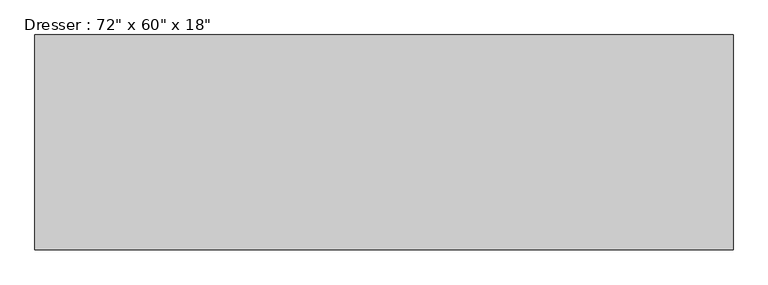
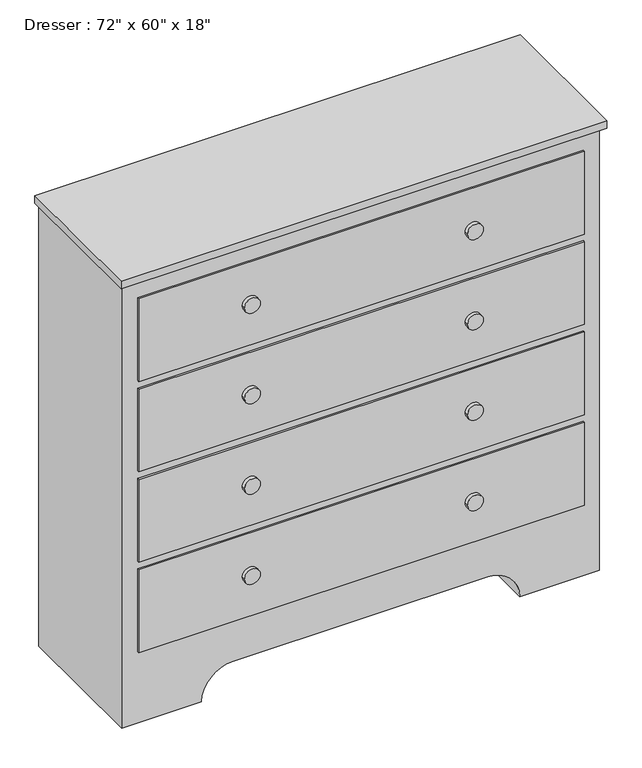
"""IFC4 building model written with IfcOpenShell, lengths in millimetres: furniture geometry."""

from ifc_helpers import new_model, si_unit, point, frame, frame_2d, origin, place, context, project, spatial, polyline, circle_curve, trimmed, segment, composite_curve, outline, extrude, source, transform, mapped, element, save


def furniture_06d35bcb(model_context):
    return source(origin(), model_context, "Body", "SweptSolid", [
        extrude(outline(polyline([(505.5067402, -134.5629541), (505.5067402, -610.8129541), (-1043.8932598, -610.8129541), (-1043.8932598, -134.5629541), (505.5067402, -134.5629541)])), frame((0.0, 0.0, 1498.6), z_axis=(0.0, 0.0, 1.0), x_axis=(1.0, 0.0, 0.0)), (0.0, 0.0, 1.0), 25.4),
        extrude(outline(composite_curve([segment(polyline([(0.0, 492.8067402), (1498.6, 492.8067402), (1498.6, -1031.1932598), (0.0, -1031.1932598), (0.0, -777.1932598)]), True, "CONTINUOUS"), segment(trimmed(circle_curve(frame_2d((0.0, -675.5932598)), 101.6), [point((0.0, -777.1932598))], [point((101.6, -675.5932598))], True, "CARTESIAN"), True, "CONTINUOUS"), segment(polyline([(101.6, -675.5932598), (101.6, 137.2067402)]), True, "CONTINUOUS"), segment(trimmed(circle_curve(frame_2d((0.0, 137.2067402)), 101.6), [point((101.6, 137.2067402))], [point((0.0, 238.8067402))], True, "CARTESIAN"), True, "CONTINUOUS"), segment(polyline([(0.0, 238.8067402), (0.0, 492.8067402)]), True, "CONTINUOUS")], self_intersect=False)), frame((0.0, -591.7629541, 0.0), z_axis=(0.0, 1.0, 0.0), x_axis=(0.0, 0.0, 1.0)), (0.0, 0.0, 1.0), 457.2),
        extrude(outline(composite_curve([segment(trimmed(circle_curve(frame_2d((1295.4, 86.4067402)), 25.4), [point((1295.4, 61.0067402))], [point((1295.4, 111.8067402))], False, "CARTESIAN"), True, "CONTINUOUS"), segment(trimmed(circle_curve(frame_2d((1295.4, 86.4067402)), 25.4), [point((1295.4, 111.8067402))], [point((1295.4, 61.0067402))], False, "CARTESIAN"), True, "CONTINUOUS")], self_intersect=False)), frame((0.0, -610.8129541, 0.0), z_axis=(0.0, 1.0, 0.0), x_axis=(0.0, 0.0, 1.0)), (0.0, 0.0, 1.0), 12.7),
        extrude(outline(composite_curve([segment(trimmed(circle_curve(frame_2d((990.6, 86.4067402)), 25.4), [point((990.6, 61.0067402))], [point((990.6, 111.8067402))], False, "CARTESIAN"), True, "CONTINUOUS"), segment(trimmed(circle_curve(frame_2d((990.6, 86.4067402)), 25.4), [point((990.6, 111.8067402))], [point((990.6, 61.0067402))], False, "CARTESIAN"), True, "CONTINUOUS")], self_intersect=False)), frame((0.0, -610.8129541, 0.0), z_axis=(0.0, 1.0, 0.0), x_axis=(0.0, 0.0, 1.0)), (0.0, 0.0, 1.0), 12.7),
        extrude(outline(composite_curve([segment(trimmed(circle_curve(frame_2d((685.8, 86.4067402)), 25.4), [point((685.8, 61.0067402))], [point((685.8, 111.8067402))], False, "CARTESIAN"), True, "CONTINUOUS"), segment(trimmed(circle_curve(frame_2d((685.8, 86.4067402)), 25.4), [point((685.8, 111.8067402))], [point((685.8, 61.0067402))], False, "CARTESIAN"), True, "CONTINUOUS")], self_intersect=False)), frame((0.0, -610.8129541, 0.0), z_axis=(0.0, 1.0, 0.0), x_axis=(0.0, 0.0, 1.0)), (0.0, 0.0, 1.0), 12.7),
        extrude(outline(composite_curve([segment(trimmed(circle_curve(frame_2d((381.0, 86.4067402)), 25.4), [point((381.0, 61.0067402))], [point((381.0, 111.8067402))], False, "CARTESIAN"), True, "CONTINUOUS"), segment(trimmed(circle_curve(frame_2d((381.0, 86.4067402)), 25.4), [point((381.0, 111.8067402))], [point((381.0, 61.0067402))], False, "CARTESIAN"), True, "CONTINUOUS")], self_intersect=False)), frame((0.0, -610.8129541, 0.0), z_axis=(0.0, 1.0, 0.0), x_axis=(0.0, 0.0, 1.0)), (0.0, 0.0, 1.0), 12.7),
        extrude(outline(composite_curve([segment(trimmed(circle_curve(frame_2d((381.0, -624.7932598)), 25.4), [point((381.0, -650.1932598))], [point((381.0, -599.3932598))], False, "CARTESIAN"), True, "CONTINUOUS"), segment(trimmed(circle_curve(frame_2d((381.0, -624.7932598)), 25.4), [point((381.0, -599.3932598))], [point((381.0, -650.1932598))], False, "CARTESIAN"), True, "CONTINUOUS")], self_intersect=False)), frame((0.0, -610.8129541, 0.0), z_axis=(0.0, 1.0, 0.0), x_axis=(0.0, 0.0, 1.0)), (0.0, 0.0, 1.0), 12.7),
        extrude(outline(composite_curve([segment(trimmed(circle_curve(frame_2d((685.8, -624.7932598)), 25.4), [point((685.8, -650.1932598))], [point((685.8, -599.3932598))], False, "CARTESIAN"), True, "CONTINUOUS"), segment(trimmed(circle_curve(frame_2d((685.8, -624.7932598)), 25.4), [point((685.8, -599.3932598))], [point((685.8, -650.1932598))], False, "CARTESIAN"), True, "CONTINUOUS")], self_intersect=False)), frame((0.0, -610.8129541, 0.0), z_axis=(0.0, 1.0, 0.0), x_axis=(0.0, 0.0, 1.0)), (0.0, 0.0, 1.0), 12.7),
        extrude(outline(composite_curve([segment(trimmed(circle_curve(frame_2d((990.6, -624.7932598)), 25.4), [point((990.6, -650.1932598))], [point((990.6, -599.3932598))], False, "CARTESIAN"), True, "CONTINUOUS"), segment(trimmed(circle_curve(frame_2d((990.6, -624.7932598)), 25.4), [point((990.6, -599.3932598))], [point((990.6, -650.1932598))], False, "CARTESIAN"), True, "CONTINUOUS")], self_intersect=False)), frame((0.0, -610.8129541, 0.0), z_axis=(0.0, 1.0, 0.0), x_axis=(0.0, 0.0, 1.0)), (0.0, 0.0, 1.0), 12.7),
        extrude(outline(composite_curve([segment(trimmed(circle_curve(frame_2d((1295.4, -624.7932598)), 25.4), [point((1295.4, -650.1932598))], [point((1295.4, -599.3932598))], False, "CARTESIAN"), True, "CONTINUOUS"), segment(trimmed(circle_curve(frame_2d((1295.4, -624.7932598)), 25.4), [point((1295.4, -599.3932598))], [point((1295.4, -650.1932598))], False, "CARTESIAN"), True, "CONTINUOUS")], self_intersect=False)), frame((0.0, -610.8129541, 0.0), z_axis=(0.0, 1.0, 0.0), x_axis=(0.0, 0.0, 1.0)), (0.0, 0.0, 1.0), 12.7),
        extrude(outline(polyline([(442.0067402, -598.1129541), (-980.3932598, -598.1129541), (-980.3932598, -591.7629541), (442.0067402, -591.7629541), (442.0067402, -598.1129541)])), frame((0.0, 0.0, 1155.7), z_axis=(0.0, 0.0, 1.0), x_axis=(1.0, 0.0, 0.0)), (0.0, 0.0, 1.0), 279.4),
        extrude(outline(polyline([(442.0067402, -598.1129541), (-980.3932598, -598.1129541), (-980.3932598, -591.7629541), (442.0067402, -591.7629541), (442.0067402, -598.1129541)])), frame((0.0, 0.0, 850.9), z_axis=(0.0, 0.0, 1.0), x_axis=(1.0, 0.0, 0.0)), (0.0, 0.0, 1.0), 279.4),
        extrude(outline(polyline([(442.0067402, -598.1129541), (-980.3932598, -598.1129541), (-980.3932598, -591.7629541), (442.0067402, -591.7629541), (442.0067402, -598.1129541)])), frame((0.0, 0.0, 546.1), z_axis=(0.0, 0.0, 1.0), x_axis=(1.0, 0.0, 0.0)), (0.0, 0.0, 1.0), 279.4),
        extrude(outline(polyline([(442.0067402, -598.1129541), (-980.3932598, -598.1129541), (-980.3932598, -591.7629541), (442.0067402, -591.7629541), (442.0067402, -598.1129541)])), frame((0.0, 0.0, 241.3), z_axis=(0.0, 0.0, 1.0), x_axis=(1.0, 0.0, 0.0)), (0.0, 0.0, 1.0), 279.4),
    ])


if __name__ == "__main__":
    model = new_model("IFC4")
    model_context = context("Model", 3, world=origin())
    ifc_project = project(units=[si_unit("LENGTHUNIT", "METRE", prefix="MILLI")], contexts=[model_context])
    site = spatial("IfcSite", under=ifc_project)
    building = spatial("IfcBuilding", under=site)
    placement = place(None, origin())
    furniture_shape = furniture_06d35bcb(model_context)
    element("IfcFurniture", 1, ObjectType="Dresser : 72\" x 60\" x 18\"", at=placement, inside=building, context=model_context, shape_type="MappedRepresentation", body=[
        mapped(furniture_shape, transform((0.0, 0.0, 0.0), x_axis=(1.0, 0.0, 0.0), y_axis=(0.0, 1.0, 0.0), z_axis=(0.0, 0.0, 1.0))),
    ])
    save(model, "model.ifc")

# Revit data of these elements
# Type "Dresser : 72\" x 60\" x 18\""
#   Assembly Code = "E2020200"
#   Depth = 1' - 6"
#   Height = 5' - 0"
#   Width = 5' - 0"
#   Dresser Material = Laminate - Ivory, Glossy
#   Drawer Material = Laminate, Ivory, Matte
#   Knob Material = Cherry
#   Default Elevation = 0
# Element 1 (IfcFurniture, "Dresser : 72\" x 60\" x 18\"")
#   Materials on its faces: "Laminate, Ivory, Matte", "Cherry", "Laminate - Ivory, Glossy"
# Materials
#   "Laminate - Ivory, Glossy": colour RGB 247 247 239, transparency 0
#   "Laminate, Ivory, Matte": class "Plastic", colour RGB 247 247 239, transparency 0, Description = "Plastic Laminate - Ivory, Matte", Cost = 0
#   "Cherry": class "Wood", colour RGB 226 177 128, transparency 0, Description = "Prunus Serotina", Cost = 0
